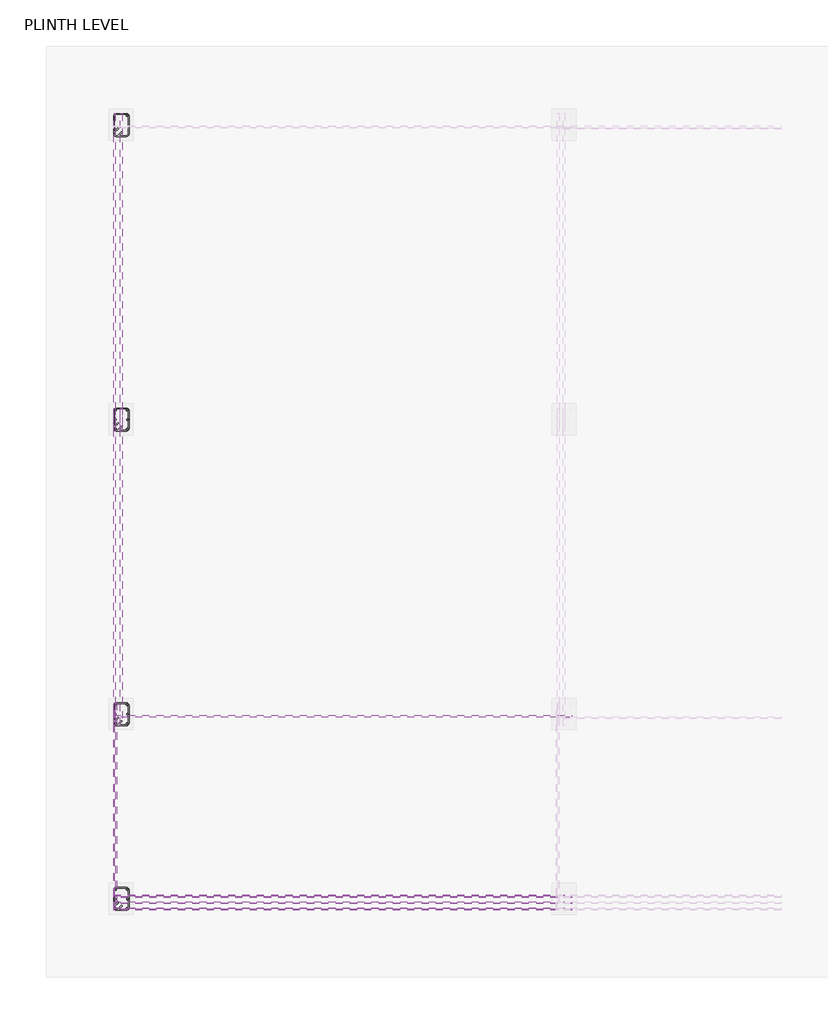
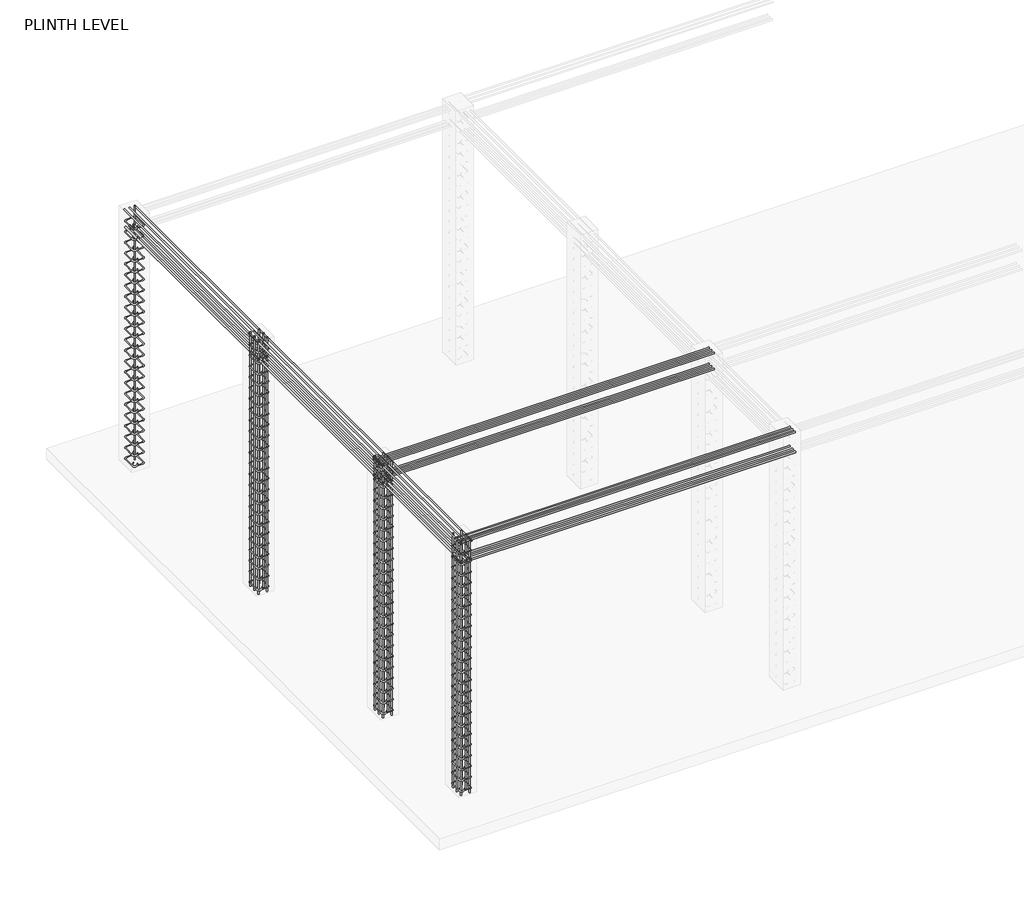
# One storey, part 2 of 6: 37 reinforcing bars.
"""IFC4 building model written with IfcOpenShell, lengths in millimetres."""

from ifc_helpers import new_model, si_unit, point, frame, origin, place, context, project, spatial, polyline, circle_curve, trimmed, segment, composite_curve, source, transform, mapped, element, save
from ifc_brep_helpers import swept_disk

model = new_model("IFC4")

# Units and contexts
model_context = context("Model", 3, world=origin())
ifc_project = project(units=[si_unit("LENGTHUNIT", "METRE", prefix="MILLI")], contexts=[model_context])

# Site, building, storey
site = spatial("IfcSite", under=ifc_project)
building = spatial("IfcBuilding", under=site)
storey = spatial("IfcBuildingStorey", under=building, Name="PLINTH LEVEL", Elevation=0.0)

# Reinforcing bars
placement = place(None, origin())
reinforcing_bar_shape = source(origin(), model_context, "Body", "SolidModel", [
    swept_disk(composite_curve([segment(polyline([(-2649.751223, -15125.7150493, 44.0), (-2683.6923485, -15159.6561748, 44.0)]), True, "CONTINUOUS"), segment(trimmed(circle_curve(frame((-2666.7217857, -15176.6267376, 44.0), z_axis=(0.0, 0.0, 1.0), x_axis=(-16.970562800000152, 16.970562799999243, 0.0)), 24.0), [point((-2683.6923485, -15159.6561748, 44.0))], [point((-2666.7217857, -15200.6267376, 44.0))], True, "CARTESIAN"), True, "CONTINUOUS"), segment(polyline([(-2666.7217857, -15200.6267376, 44.0), (-2572.7217857, -15200.6267376, 44.0)]), True, "CONTINUOUS"), segment(trimmed(circle_curve(frame((-2572.7217857, -15176.6267376, 44.0), z_axis=(0.0, 0.0, 1.0), x_axis=(0.0, -24.0, 0.0)), 24.0), [point((-2572.7217857, -15200.6267376, 44.0))], [point((-2548.7217857, -15176.6267376, 44.0))], True, "CARTESIAN"), True, "CONTINUOUS"), segment(polyline([(-2548.7217857, -15176.6267376, 44.0), (-2548.7217857, -15012.6267376, 44.0)]), True, "CONTINUOUS"), segment(trimmed(circle_curve(frame((-2572.6837885, -15012.6267376, 42.650028), z_axis=(-0.05624883273897079, 0.0, 0.9984167811167355), x_axis=(23.962002799999937, 0.0, 1.349972000000001)), 24.0), [point((-2548.7217857, -15012.6267376, 44.0))], [point((-2572.6837885, -14988.6267376, 42.650028))], True, "CARTESIAN"), True, "CONTINUOUS"), segment(polyline([(-2572.6837885, -14988.6267376, 42.650028), (-2666.759783, -14988.6267376, 37.349972)]), True, "CONTINUOUS"), segment(trimmed(circle_curve(frame((-2666.759783, -15012.6267376, 37.349972), z_axis=(-0.05624883273897079, 0.0, 0.9984167811167355), x_axis=(0.0, 24.0, 0.0)), 24.0), [point((-2666.759783, -14988.6267376, 37.349972))], [point((-2690.7217857, -15012.6267376, 36.0))], True, "CARTESIAN"), True, "CONTINUOUS"), segment(polyline([(-2690.7217857, -15012.6267376, 36.0), (-2690.7217857, -15176.6267376, 36.0)]), True, "CONTINUOUS"), segment(trimmed(circle_curve(frame((-2666.7217857, -15176.6267376, 36.0), z_axis=(0.0, 0.0, 1.0), x_axis=(-24.0, 0.0, 0.0)), 24.0), [point((-2690.7217857, -15176.6267376, 36.0))], [point((-2649.751223, -15193.5973003, 36.0))], True, "CARTESIAN"), True, "CONTINUOUS"), segment(polyline([(-2649.751223, -15193.5973003, 36.0), (-2615.8100975, -15159.6561748, 36.0)]), True, "CONTINUOUS")], self_intersect=False), 4.0),
])
element("IfcReinforcingBar", 1, at=placement, inside=storey, context=model_context, shape_type="MappedRepresentation", body=[
    mapped(reinforcing_bar_shape, transform((0.0, 0.0, 0.0), x_axis=(1.0, 0.0, 0.0), y_axis=(0.0, 1.0, 0.0), z_axis=(0.0, 0.0, 1.0))),
    mapped(reinforcing_bar_shape, transform((0.0, 0.0, 149.0483786), x_axis=(1.0, 0.0, 0.0), y_axis=(0.0, 1.0, 0.0), z_axis=(0.0, 0.0, 1.0))),
    mapped(reinforcing_bar_shape, transform((0.0, 0.0, 298.0967572), x_axis=(1.0, 0.0, 0.0), y_axis=(0.0, 1.0, 0.0), z_axis=(0.0, 0.0, 1.0))),
    mapped(reinforcing_bar_shape, transform((0.0, 0.0, 447.1451358), x_axis=(1.0, 0.0, 0.0), y_axis=(0.0, 1.0, 0.0), z_axis=(0.0, 0.0, 1.0))),
    mapped(reinforcing_bar_shape, transform((0.0, 0.0, 596.1935144), x_axis=(1.0, 0.0, 0.0), y_axis=(0.0, 1.0, 0.0), z_axis=(0.0, 0.0, 1.0))),
    mapped(reinforcing_bar_shape, transform((0.0, 0.0, 745.241893), x_axis=(1.0, 0.0, 0.0), y_axis=(0.0, 1.0, 0.0), z_axis=(0.0, 0.0, 1.0))),
    mapped(reinforcing_bar_shape, transform((0.0, 0.0, 894.2902717), x_axis=(1.0, 0.0, 0.0), y_axis=(0.0, 1.0, 0.0), z_axis=(0.0, 0.0, 1.0))),
    mapped(reinforcing_bar_shape, transform((0.0, 0.0, 1043.3386503), x_axis=(1.0, 0.0, 0.0), y_axis=(0.0, 1.0, 0.0), z_axis=(0.0, 0.0, 1.0))),
    mapped(reinforcing_bar_shape, transform((0.0, 0.0, 1192.3870289), x_axis=(1.0, 0.0, 0.0), y_axis=(0.0, 1.0, 0.0), z_axis=(0.0, 0.0, 1.0))),
    mapped(reinforcing_bar_shape, transform((0.0, 0.0, 1341.4354075), x_axis=(1.0, 0.0, 0.0), y_axis=(0.0, 1.0, 0.0), z_axis=(0.0, 0.0, 1.0))),
    mapped(reinforcing_bar_shape, transform((0.0, 0.0, 1490.4837861), x_axis=(1.0, 0.0, 0.0), y_axis=(0.0, 1.0, 0.0), z_axis=(0.0, 0.0, 1.0))),
    mapped(reinforcing_bar_shape, transform((0.0, 0.0, 1639.5321647), x_axis=(1.0, 0.0, 0.0), y_axis=(0.0, 1.0, 0.0), z_axis=(0.0, 0.0, 1.0))),
    mapped(reinforcing_bar_shape, transform((0.0, 0.0, 1788.5805433), x_axis=(1.0, 0.0, 0.0), y_axis=(0.0, 1.0, 0.0), z_axis=(0.0, 0.0, 1.0))),
    mapped(reinforcing_bar_shape, transform((0.0, 0.0, 1937.6289219), x_axis=(1.0, 0.0, 0.0), y_axis=(0.0, 1.0, 0.0), z_axis=(0.0, 0.0, 1.0))),
    mapped(reinforcing_bar_shape, transform((0.0, 0.0, 2086.6773005), x_axis=(1.0, 0.0, 0.0), y_axis=(0.0, 1.0, 0.0), z_axis=(0.0, 0.0, 1.0))),
    mapped(reinforcing_bar_shape, transform((0.0, 0.0, 2235.7256791), x_axis=(1.0, 0.0, 0.0), y_axis=(0.0, 1.0, 0.0), z_axis=(0.0, 0.0, 1.0))),
    mapped(reinforcing_bar_shape, transform((0.0, 0.0, 2384.7740578), x_axis=(1.0, 0.0, 0.0), y_axis=(0.0, 1.0, 0.0), z_axis=(0.0, 0.0, 1.0))),
    mapped(reinforcing_bar_shape, transform((0.0, 0.0, 2533.8224364), x_axis=(1.0, 0.0, 0.0), y_axis=(0.0, 1.0, 0.0), z_axis=(0.0, 0.0, 1.0))),
    mapped(reinforcing_bar_shape, transform((0.0, 0.0, 2682.870815), x_axis=(1.0, 0.0, 0.0), y_axis=(0.0, 1.0, 0.0), z_axis=(0.0, 0.0, 1.0))),
    mapped(reinforcing_bar_shape, transform((0.0, 0.0, 2831.9191936), x_axis=(1.0, 0.0, 0.0), y_axis=(0.0, 1.0, 0.0), z_axis=(0.0, 0.0, 1.0))),
    mapped(reinforcing_bar_shape, transform((0.0, 0.0, 2980.9675722), x_axis=(1.0, 0.0, 0.0), y_axis=(0.0, 1.0, 0.0), z_axis=(0.0, 0.0, 1.0))),
    mapped(reinforcing_bar_shape, transform((0.0, 0.0, 3130.0159508), x_axis=(1.0, 0.0, 0.0), y_axis=(0.0, 1.0, 0.0), z_axis=(0.0, 0.0, 1.0))),
    mapped(reinforcing_bar_shape, transform((0.0, 0.0, 3279.0643294), x_axis=(1.0, 0.0, 0.0), y_axis=(0.0, 1.0, 0.0), z_axis=(0.0, 0.0, 1.0))),
])
element("IfcReinforcingBar", 2, at=placement, inside=storey, context=model_context, shape_type="SolidModel", body=[
    swept_disk(composite_curve([segment(polyline([(-2564.2365043, -15004.1414562, -20.0), (-2564.2365043, -15004.1414562, 3485.2)]), True, "CONTINUOUS")], self_intersect=False), 8.0),
])
element("IfcReinforcingBar", 3, at=placement, inside=storey, context=model_context, shape_type="SolidModel", body=[
    swept_disk(composite_curve([segment(polyline([(-2564.2365043, -15185.112019, -20.0), (-2564.2365043, -15185.112019, 3485.2)]), True, "CONTINUOUS")], self_intersect=False), 8.0),
])
element("IfcReinforcingBar", 4, at=placement, inside=storey, context=model_context, shape_type="SolidModel", body=[
    swept_disk(composite_curve([segment(polyline([(-2560.7217857, -15094.6267376, -20.0), (-2560.7217857, -15094.6267376, 3485.2)]), True, "CONTINUOUS")], self_intersect=False), 8.0),
])
element("IfcReinforcingBar", 5, at=placement, inside=storey, context=model_context, shape_type="SolidModel", body=[
    swept_disk(composite_curve([segment(polyline([(-2675.2070671, -15004.1414562, -20.0), (-2675.2070671, -15004.1414562, 3485.2)]), True, "CONTINUOUS")], self_intersect=False), 8.0),
])
element("IfcReinforcingBar", 6, at=placement, inside=storey, context=model_context, shape_type="SolidModel", body=[
    swept_disk(composite_curve([segment(polyline([(-2675.2070671, -15185.112019, -20.0), (-2675.2070671, -15185.112019, 3485.2)]), True, "CONTINUOUS")], self_intersect=False), 8.0),
])
element("IfcReinforcingBar", 7, at=placement, inside=storey, context=model_context, shape_type="SolidModel", body=[
    swept_disk(composite_curve([segment(polyline([(-2678.7217857, -15094.6267376, -20.0), (-2678.7217857, -15094.6267376, 3485.2)]), True, "CONTINUOUS")], self_intersect=False), 8.0),
])
reinforcing_bar_2_shape = source(origin(), model_context, "Body", "SolidModel", [
    swept_disk(composite_curve([segment(polyline([(-2649.751223, -13360.7150493, 44.0), (-2683.6923485, -13394.6561748, 44.0)]), True, "CONTINUOUS"), segment(trimmed(circle_curve(frame((-2666.7217857, -13411.6267376, 44.0), z_axis=(0.0, 0.0, 1.0), x_axis=(-16.970562800000152, 16.970562799999243, 0.0)), 24.0), [point((-2683.6923485, -13394.6561748, 44.0))], [point((-2666.7217857, -13435.6267376, 44.0))], True, "CARTESIAN"), True, "CONTINUOUS"), segment(polyline([(-2666.7217857, -13435.6267376, 44.0), (-2572.7217857, -13435.6267376, 44.0)]), True, "CONTINUOUS"), segment(trimmed(circle_curve(frame((-2572.7217857, -13411.6267376, 44.0), z_axis=(0.0, 0.0, 1.0), x_axis=(0.0, -24.0, 0.0)), 24.0), [point((-2572.7217857, -13435.6267376, 44.0))], [point((-2548.7217857, -13411.6267376, 44.0))], True, "CARTESIAN"), True, "CONTINUOUS"), segment(polyline([(-2548.7217857, -13411.6267376, 44.0), (-2548.7217857, -13247.6267376, 44.0)]), True, "CONTINUOUS"), segment(trimmed(circle_curve(frame((-2572.6837885, -13247.6267376, 42.650028), z_axis=(-0.05624883273897079, 0.0, 0.9984167811167355), x_axis=(23.962002799999937, 0.0, 1.349972000000001)), 24.0), [point((-2548.7217857, -13247.6267376, 44.0))], [point((-2572.6837885, -13223.6267376, 42.650028))], True, "CARTESIAN"), True, "CONTINUOUS"), segment(polyline([(-2572.6837885, -13223.6267376, 42.650028), (-2666.759783, -13223.6267376, 37.349972)]), True, "CONTINUOUS"), segment(trimmed(circle_curve(frame((-2666.759783, -13247.6267376, 37.349972), z_axis=(-0.05624883273897079, 0.0, 0.9984167811167355), x_axis=(0.0, 24.0, 0.0)), 24.0), [point((-2666.759783, -13223.6267376, 37.349972))], [point((-2690.7217857, -13247.6267376, 36.0))], True, "CARTESIAN"), True, "CONTINUOUS"), segment(polyline([(-2690.7217857, -13247.6267376, 36.0), (-2690.7217857, -13411.6267376, 36.0)]), True, "CONTINUOUS"), segment(trimmed(circle_curve(frame((-2666.7217857, -13411.6267376, 36.0), z_axis=(0.0, 0.0, 1.0), x_axis=(-24.0, 0.0, 0.0)), 24.0), [point((-2690.7217857, -13411.6267376, 36.0))], [point((-2649.751223, -13428.5973003, 36.0))], True, "CARTESIAN"), True, "CONTINUOUS"), segment(polyline([(-2649.751223, -13428.5973003, 36.0), (-2615.8100975, -13394.6561748, 36.0)]), True, "CONTINUOUS")], self_intersect=False), 4.0),
])
element("IfcReinforcingBar", 8, at=placement, inside=storey, context=model_context, shape_type="MappedRepresentation", body=[
    mapped(reinforcing_bar_2_shape, transform((0.0, 0.0, 0.0), x_axis=(1.0, 0.0, 0.0), y_axis=(0.0, 1.0, 0.0), z_axis=(0.0, 0.0, 1.0))),
    mapped(reinforcing_bar_2_shape, transform((0.0, 0.0, 149.0483786), x_axis=(1.0, 0.0, 0.0), y_axis=(0.0, 1.0, 0.0), z_axis=(0.0, 0.0, 1.0))),
    mapped(reinforcing_bar_2_shape, transform((0.0, 0.0, 298.0967572), x_axis=(1.0, 0.0, 0.0), y_axis=(0.0, 1.0, 0.0), z_axis=(0.0, 0.0, 1.0))),
    mapped(reinforcing_bar_2_shape, transform((0.0, 0.0, 447.1451358), x_axis=(1.0, 0.0, 0.0), y_axis=(0.0, 1.0, 0.0), z_axis=(0.0, 0.0, 1.0))),
    mapped(reinforcing_bar_2_shape, transform((0.0, 0.0, 596.1935144), x_axis=(1.0, 0.0, 0.0), y_axis=(0.0, 1.0, 0.0), z_axis=(0.0, 0.0, 1.0))),
    mapped(reinforcing_bar_2_shape, transform((0.0, 0.0, 745.241893), x_axis=(1.0, 0.0, 0.0), y_axis=(0.0, 1.0, 0.0), z_axis=(0.0, 0.0, 1.0))),
    mapped(reinforcing_bar_2_shape, transform((0.0, 0.0, 894.2902717), x_axis=(1.0, 0.0, 0.0), y_axis=(0.0, 1.0, 0.0), z_axis=(0.0, 0.0, 1.0))),
    mapped(reinforcing_bar_2_shape, transform((0.0, 0.0, 1043.3386503), x_axis=(1.0, 0.0, 0.0), y_axis=(0.0, 1.0, 0.0), z_axis=(0.0, 0.0, 1.0))),
    mapped(reinforcing_bar_2_shape, transform((0.0, 0.0, 1192.3870289), x_axis=(1.0, 0.0, 0.0), y_axis=(0.0, 1.0, 0.0), z_axis=(0.0, 0.0, 1.0))),
    mapped(reinforcing_bar_2_shape, transform((0.0, 0.0, 1341.4354075), x_axis=(1.0, 0.0, 0.0), y_axis=(0.0, 1.0, 0.0), z_axis=(0.0, 0.0, 1.0))),
    mapped(reinforcing_bar_2_shape, transform((0.0, 0.0, 1490.4837861), x_axis=(1.0, 0.0, 0.0), y_axis=(0.0, 1.0, 0.0), z_axis=(0.0, 0.0, 1.0))),
    mapped(reinforcing_bar_2_shape, transform((0.0, 0.0, 1639.5321647), x_axis=(1.0, 0.0, 0.0), y_axis=(0.0, 1.0, 0.0), z_axis=(0.0, 0.0, 1.0))),
    mapped(reinforcing_bar_2_shape, transform((0.0, 0.0, 1788.5805433), x_axis=(1.0, 0.0, 0.0), y_axis=(0.0, 1.0, 0.0), z_axis=(0.0, 0.0, 1.0))),
    mapped(reinforcing_bar_2_shape, transform((0.0, 0.0, 1937.6289219), x_axis=(1.0, 0.0, 0.0), y_axis=(0.0, 1.0, 0.0), z_axis=(0.0, 0.0, 1.0))),
    mapped(reinforcing_bar_2_shape, transform((0.0, 0.0, 2086.6773005), x_axis=(1.0, 0.0, 0.0), y_axis=(0.0, 1.0, 0.0), z_axis=(0.0, 0.0, 1.0))),
    mapped(reinforcing_bar_2_shape, transform((0.0, 0.0, 2235.7256791), x_axis=(1.0, 0.0, 0.0), y_axis=(0.0, 1.0, 0.0), z_axis=(0.0, 0.0, 1.0))),
    mapped(reinforcing_bar_2_shape, transform((0.0, 0.0, 2384.7740578), x_axis=(1.0, 0.0, 0.0), y_axis=(0.0, 1.0, 0.0), z_axis=(0.0, 0.0, 1.0))),
    mapped(reinforcing_bar_2_shape, transform((0.0, 0.0, 2533.8224364), x_axis=(1.0, 0.0, 0.0), y_axis=(0.0, 1.0, 0.0), z_axis=(0.0, 0.0, 1.0))),
    mapped(reinforcing_bar_2_shape, transform((0.0, 0.0, 2682.870815), x_axis=(1.0, 0.0, 0.0), y_axis=(0.0, 1.0, 0.0), z_axis=(0.0, 0.0, 1.0))),
    mapped(reinforcing_bar_2_shape, transform((0.0, 0.0, 2831.9191936), x_axis=(1.0, 0.0, 0.0), y_axis=(0.0, 1.0, 0.0), z_axis=(0.0, 0.0, 1.0))),
    mapped(reinforcing_bar_2_shape, transform((0.0, 0.0, 2980.9675722), x_axis=(1.0, 0.0, 0.0), y_axis=(0.0, 1.0, 0.0), z_axis=(0.0, 0.0, 1.0))),
    mapped(reinforcing_bar_2_shape, transform((0.0, 0.0, 3130.0159508), x_axis=(1.0, 0.0, 0.0), y_axis=(0.0, 1.0, 0.0), z_axis=(0.0, 0.0, 1.0))),
    mapped(reinforcing_bar_2_shape, transform((0.0, 0.0, 3279.0643294), x_axis=(1.0, 0.0, 0.0), y_axis=(0.0, 1.0, 0.0), z_axis=(0.0, 0.0, 1.0))),
])
element("IfcReinforcingBar", 9, at=placement, inside=storey, context=model_context, shape_type="SolidModel", body=[
    swept_disk(composite_curve([segment(polyline([(-2564.2365043, -13239.1414562, -20.0), (-2564.2365043, -13239.1414562, 3485.2)]), True, "CONTINUOUS")], self_intersect=False), 8.0),
])
element("IfcReinforcingBar", 10, at=placement, inside=storey, context=model_context, shape_type="SolidModel", body=[
    swept_disk(composite_curve([segment(polyline([(-2564.2365043, -13420.112019, -20.0), (-2564.2365043, -13420.112019, 3485.2)]), True, "CONTINUOUS")], self_intersect=False), 8.0),
])
element("IfcReinforcingBar", 11, at=placement, inside=storey, context=model_context, shape_type="SolidModel", body=[
    swept_disk(composite_curve([segment(polyline([(-2560.7217857, -13329.6267376, -20.0), (-2560.7217857, -13329.6267376, 3485.2)]), True, "CONTINUOUS")], self_intersect=False), 8.0),
])
element("IfcReinforcingBar", 12, at=placement, inside=storey, context=model_context, shape_type="SolidModel", body=[
    swept_disk(composite_curve([segment(polyline([(-2675.2070671, -13239.1414562, -20.0), (-2675.2070671, -13239.1414562, 3485.2)]), True, "CONTINUOUS")], self_intersect=False), 8.0),
])
element("IfcReinforcingBar", 13, at=placement, inside=storey, context=model_context, shape_type="SolidModel", body=[
    swept_disk(composite_curve([segment(polyline([(-2675.2070671, -13420.112019, -20.0), (-2675.2070671, -13420.112019, 3485.2)]), True, "CONTINUOUS")], self_intersect=False), 8.0),
])
element("IfcReinforcingBar", 14, at=placement, inside=storey, context=model_context, shape_type="SolidModel", body=[
    swept_disk(composite_curve([segment(polyline([(-2678.7217857, -13329.6267376, -20.0), (-2678.7217857, -13329.6267376, 3485.2)]), True, "CONTINUOUS")], self_intersect=False), 8.0),
])
reinforcing_bar_3_shape = source(origin(), model_context, "Body", "SolidModel", [
    swept_disk(composite_curve([segment(polyline([(-2649.751223, -10545.7150493, 44.0), (-2683.6923485, -10579.6561748, 44.0)]), True, "CONTINUOUS"), segment(trimmed(circle_curve(frame((-2666.7217857, -10596.6267376, 44.0), z_axis=(0.0, 0.0, 1.0), x_axis=(-16.970562800000152, 16.970562799999243, 0.0)), 24.0), [point((-2683.6923485, -10579.6561748, 44.0))], [point((-2666.7217857, -10620.6267376, 44.0))], True, "CARTESIAN"), True, "CONTINUOUS"), segment(polyline([(-2666.7217857, -10620.6267376, 44.0), (-2572.7217857, -10620.6267376, 44.0)]), True, "CONTINUOUS"), segment(trimmed(circle_curve(frame((-2572.7217857, -10596.6267376, 44.0), z_axis=(0.0, 0.0, 1.0), x_axis=(0.0, -24.0, 0.0)), 24.0), [point((-2572.7217857, -10620.6267376, 44.0))], [point((-2548.7217857, -10596.6267376, 44.0))], True, "CARTESIAN"), True, "CONTINUOUS"), segment(polyline([(-2548.7217857, -10596.6267376, 44.0), (-2548.7217857, -10432.6267376, 44.0)]), True, "CONTINUOUS"), segment(trimmed(circle_curve(frame((-2572.6837885, -10432.6267376, 42.650028), z_axis=(-0.05624883273897079, 0.0, 0.9984167811167355), x_axis=(23.962002799999937, 0.0, 1.349972000000001)), 24.0), [point((-2548.7217857, -10432.6267376, 44.0))], [point((-2572.6837885, -10408.6267376, 42.650028))], True, "CARTESIAN"), True, "CONTINUOUS"), segment(polyline([(-2572.6837885, -10408.6267376, 42.650028), (-2666.759783, -10408.6267376, 37.349972)]), True, "CONTINUOUS"), segment(trimmed(circle_curve(frame((-2666.759783, -10432.6267376, 37.349972), z_axis=(-0.05624883273897079, 0.0, 0.9984167811167355), x_axis=(0.0, 24.0, 0.0)), 24.0), [point((-2666.759783, -10408.6267376, 37.349972))], [point((-2690.7217857, -10432.6267376, 36.0))], True, "CARTESIAN"), True, "CONTINUOUS"), segment(polyline([(-2690.7217857, -10432.6267376, 36.0), (-2690.7217857, -10596.6267376, 36.0)]), True, "CONTINUOUS"), segment(trimmed(circle_curve(frame((-2666.7217857, -10596.6267376, 36.0), z_axis=(0.0, 0.0, 1.0), x_axis=(-24.0, 0.0, 0.0)), 24.0), [point((-2690.7217857, -10596.6267376, 36.0))], [point((-2649.751223, -10613.5973003, 36.0))], True, "CARTESIAN"), True, "CONTINUOUS"), segment(polyline([(-2649.751223, -10613.5973003, 36.0), (-2615.8100975, -10579.6561748, 36.0)]), True, "CONTINUOUS")], self_intersect=False), 4.0),
])
element("IfcReinforcingBar", 15, at=placement, inside=storey, context=model_context, shape_type="MappedRepresentation", body=[
    mapped(reinforcing_bar_3_shape, transform((0.0, 0.0, 0.0), x_axis=(1.0, 0.0, 0.0), y_axis=(0.0, 1.0, 0.0), z_axis=(0.0, 0.0, 1.0))),
    mapped(reinforcing_bar_3_shape, transform((0.0, 0.0, 149.0483786), x_axis=(1.0, 0.0, 0.0), y_axis=(0.0, 1.0, 0.0), z_axis=(0.0, 0.0, 1.0))),
    mapped(reinforcing_bar_3_shape, transform((0.0, 0.0, 298.0967572), x_axis=(1.0, 0.0, 0.0), y_axis=(0.0, 1.0, 0.0), z_axis=(0.0, 0.0, 1.0))),
    mapped(reinforcing_bar_3_shape, transform((0.0, 0.0, 447.1451358), x_axis=(1.0, 0.0, 0.0), y_axis=(0.0, 1.0, 0.0), z_axis=(0.0, 0.0, 1.0))),
    mapped(reinforcing_bar_3_shape, transform((0.0, 0.0, 596.1935144), x_axis=(1.0, 0.0, 0.0), y_axis=(0.0, 1.0, 0.0), z_axis=(0.0, 0.0, 1.0))),
    mapped(reinforcing_bar_3_shape, transform((0.0, 0.0, 745.241893), x_axis=(1.0, 0.0, 0.0), y_axis=(0.0, 1.0, 0.0), z_axis=(0.0, 0.0, 1.0))),
    mapped(reinforcing_bar_3_shape, transform((0.0, 0.0, 894.2902717), x_axis=(1.0, 0.0, 0.0), y_axis=(0.0, 1.0, 0.0), z_axis=(0.0, 0.0, 1.0))),
    mapped(reinforcing_bar_3_shape, transform((0.0, 0.0, 1043.3386503), x_axis=(1.0, 0.0, 0.0), y_axis=(0.0, 1.0, 0.0), z_axis=(0.0, 0.0, 1.0))),
    mapped(reinforcing_bar_3_shape, transform((0.0, 0.0, 1192.3870289), x_axis=(1.0, 0.0, 0.0), y_axis=(0.0, 1.0, 0.0), z_axis=(0.0, 0.0, 1.0))),
    mapped(reinforcing_bar_3_shape, transform((0.0, 0.0, 1341.4354075), x_axis=(1.0, 0.0, 0.0), y_axis=(0.0, 1.0, 0.0), z_axis=(0.0, 0.0, 1.0))),
    mapped(reinforcing_bar_3_shape, transform((0.0, 0.0, 1490.4837861), x_axis=(1.0, 0.0, 0.0), y_axis=(0.0, 1.0, 0.0), z_axis=(0.0, 0.0, 1.0))),
    mapped(reinforcing_bar_3_shape, transform((0.0, 0.0, 1639.5321647), x_axis=(1.0, 0.0, 0.0), y_axis=(0.0, 1.0, 0.0), z_axis=(0.0, 0.0, 1.0))),
    mapped(reinforcing_bar_3_shape, transform((0.0, 0.0, 1788.5805433), x_axis=(1.0, 0.0, 0.0), y_axis=(0.0, 1.0, 0.0), z_axis=(0.0, 0.0, 1.0))),
    mapped(reinforcing_bar_3_shape, transform((0.0, 0.0, 1937.6289219), x_axis=(1.0, 0.0, 0.0), y_axis=(0.0, 1.0, 0.0), z_axis=(0.0, 0.0, 1.0))),
    mapped(reinforcing_bar_3_shape, transform((0.0, 0.0, 2086.6773005), x_axis=(1.0, 0.0, 0.0), y_axis=(0.0, 1.0, 0.0), z_axis=(0.0, 0.0, 1.0))),
    mapped(reinforcing_bar_3_shape, transform((0.0, 0.0, 2235.7256791), x_axis=(1.0, 0.0, 0.0), y_axis=(0.0, 1.0, 0.0), z_axis=(0.0, 0.0, 1.0))),
    mapped(reinforcing_bar_3_shape, transform((0.0, 0.0, 2384.7740578), x_axis=(1.0, 0.0, 0.0), y_axis=(0.0, 1.0, 0.0), z_axis=(0.0, 0.0, 1.0))),
    mapped(reinforcing_bar_3_shape, transform((0.0, 0.0, 2533.8224364), x_axis=(1.0, 0.0, 0.0), y_axis=(0.0, 1.0, 0.0), z_axis=(0.0, 0.0, 1.0))),
    mapped(reinforcing_bar_3_shape, transform((0.0, 0.0, 2682.870815), x_axis=(1.0, 0.0, 0.0), y_axis=(0.0, 1.0, 0.0), z_axis=(0.0, 0.0, 1.0))),
    mapped(reinforcing_bar_3_shape, transform((0.0, 0.0, 2831.9191936), x_axis=(1.0, 0.0, 0.0), y_axis=(0.0, 1.0, 0.0), z_axis=(0.0, 0.0, 1.0))),
    mapped(reinforcing_bar_3_shape, transform((0.0, 0.0, 2980.9675722), x_axis=(1.0, 0.0, 0.0), y_axis=(0.0, 1.0, 0.0), z_axis=(0.0, 0.0, 1.0))),
    mapped(reinforcing_bar_3_shape, transform((0.0, 0.0, 3130.0159508), x_axis=(1.0, 0.0, 0.0), y_axis=(0.0, 1.0, 0.0), z_axis=(0.0, 0.0, 1.0))),
    mapped(reinforcing_bar_3_shape, transform((0.0, 0.0, 3279.0643294), x_axis=(1.0, 0.0, 0.0), y_axis=(0.0, 1.0, 0.0), z_axis=(0.0, 0.0, 1.0))),
])
element("IfcReinforcingBar", 16, at=placement, inside=storey, context=model_context, shape_type="SolidModel", body=[
    swept_disk(composite_curve([segment(polyline([(-2564.2365043, -10424.1414562, -20.0), (-2564.2365043, -10424.1414562, 3485.2)]), True, "CONTINUOUS")], self_intersect=False), 8.0),
])
element("IfcReinforcingBar", 17, at=placement, inside=storey, context=model_context, shape_type="SolidModel", body=[
    swept_disk(composite_curve([segment(polyline([(-2564.2365043, -10605.112019, -20.0), (-2564.2365043, -10605.112019, 3485.2)]), True, "CONTINUOUS")], self_intersect=False), 8.0),
])
element("IfcReinforcingBar", 18, at=placement, inside=storey, context=model_context, shape_type="SolidModel", body=[
    swept_disk(composite_curve([segment(polyline([(-2560.7217857, -10514.6267376, -20.0), (-2560.7217857, -10514.6267376, 3485.2)]), True, "CONTINUOUS")], self_intersect=False), 8.0),
])
element("IfcReinforcingBar", 19, at=placement, inside=storey, context=model_context, shape_type="SolidModel", body=[
    swept_disk(composite_curve([segment(polyline([(-2675.2070671, -10424.1414562, -20.0), (-2675.2070671, -10424.1414562, 3485.2)]), True, "CONTINUOUS")], self_intersect=False), 8.0),
])
element("IfcReinforcingBar", 20, at=placement, inside=storey, context=model_context, shape_type="SolidModel", body=[
    swept_disk(composite_curve([segment(polyline([(-2675.2070671, -10605.112019, -20.0), (-2675.2070671, -10605.112019, 3485.2)]), True, "CONTINUOUS")], self_intersect=False), 8.0),
])
element("IfcReinforcingBar", 21, at=placement, inside=storey, context=model_context, shape_type="SolidModel", body=[
    swept_disk(composite_curve([segment(polyline([(-2678.7217857, -10514.6267376, -20.0), (-2678.7217857, -10514.6267376, 3485.2)]), True, "CONTINUOUS")], self_intersect=False), 8.0),
])
reinforcing_bar_4_shape = source(origin(), model_context, "Body", "SolidModel", [
    swept_disk(composite_curve([segment(polyline([(-2649.751223, -7730.7150493, 44.0), (-2683.6923485, -7764.6561748, 44.0)]), True, "CONTINUOUS"), segment(trimmed(circle_curve(frame((-2666.7217857, -7781.6267376, 44.0), z_axis=(0.0, 0.0, 1.0), x_axis=(-16.970562800000152, 16.970562799999243, 0.0)), 24.0), [point((-2683.6923485, -7764.6561748, 44.0))], [point((-2666.7217857, -7805.6267376, 44.0))], True, "CARTESIAN"), True, "CONTINUOUS"), segment(polyline([(-2666.7217857, -7805.6267376, 44.0), (-2572.7217857, -7805.6267376, 44.0)]), True, "CONTINUOUS"), segment(trimmed(circle_curve(frame((-2572.7217857, -7781.6267376, 44.0), z_axis=(0.0, 0.0, 1.0), x_axis=(0.0, -24.0, 0.0)), 24.0), [point((-2572.7217857, -7805.6267376, 44.0))], [point((-2548.7217857, -7781.6267376, 44.0))], True, "CARTESIAN"), True, "CONTINUOUS"), segment(polyline([(-2548.7217857, -7781.6267376, 44.0), (-2548.7217857, -7617.6267376, 44.0)]), True, "CONTINUOUS"), segment(trimmed(circle_curve(frame((-2572.6837885, -7617.6267376, 42.650028), z_axis=(-0.05624883273897079, 0.0, 0.9984167811167355), x_axis=(23.962002799999937, 0.0, 1.349972000000001)), 24.0), [point((-2548.7217857, -7617.6267376, 44.0))], [point((-2572.6837885, -7593.6267376, 42.650028))], True, "CARTESIAN"), True, "CONTINUOUS"), segment(polyline([(-2572.6837885, -7593.6267376, 42.650028), (-2666.759783, -7593.6267376, 37.349972)]), True, "CONTINUOUS"), segment(trimmed(circle_curve(frame((-2666.759783, -7617.6267376, 37.349972), z_axis=(-0.05624883273897079, 0.0, 0.9984167811167355), x_axis=(0.0, 24.0, 0.0)), 24.0), [point((-2666.759783, -7593.6267376, 37.349972))], [point((-2690.7217857, -7617.6267376, 36.0))], True, "CARTESIAN"), True, "CONTINUOUS"), segment(polyline([(-2690.7217857, -7617.6267376, 36.0), (-2690.7217857, -7781.6267376, 36.0)]), True, "CONTINUOUS"), segment(trimmed(circle_curve(frame((-2666.7217857, -7781.6267376, 36.0), z_axis=(0.0, 0.0, 1.0), x_axis=(-24.0, 0.0, 0.0)), 24.0), [point((-2690.7217857, -7781.6267376, 36.0))], [point((-2649.751223, -7798.5973003, 36.0))], True, "CARTESIAN"), True, "CONTINUOUS"), segment(polyline([(-2649.751223, -7798.5973003, 36.0), (-2615.8100975, -7764.6561748, 36.0)]), True, "CONTINUOUS")], self_intersect=False), 4.0),
])
element("IfcReinforcingBar", 22, at=placement, inside=storey, context=model_context, shape_type="MappedRepresentation", body=[
    mapped(reinforcing_bar_4_shape, transform((0.0, 0.0, 0.0), x_axis=(1.0, 0.0, 0.0), y_axis=(0.0, 1.0, 0.0), z_axis=(0.0, 0.0, 1.0))),
    mapped(reinforcing_bar_4_shape, transform((0.0, 0.0, 149.0483786), x_axis=(1.0, 0.0, 0.0), y_axis=(0.0, 1.0, 0.0), z_axis=(0.0, 0.0, 1.0))),
    mapped(reinforcing_bar_4_shape, transform((0.0, 0.0, 298.0967572), x_axis=(1.0, 0.0, 0.0), y_axis=(0.0, 1.0, 0.0), z_axis=(0.0, 0.0, 1.0))),
    mapped(reinforcing_bar_4_shape, transform((0.0, 0.0, 447.1451358), x_axis=(1.0, 0.0, 0.0), y_axis=(0.0, 1.0, 0.0), z_axis=(0.0, 0.0, 1.0))),
    mapped(reinforcing_bar_4_shape, transform((0.0, 0.0, 596.1935144), x_axis=(1.0, 0.0, 0.0), y_axis=(0.0, 1.0, 0.0), z_axis=(0.0, 0.0, 1.0))),
    mapped(reinforcing_bar_4_shape, transform((0.0, 0.0, 745.241893), x_axis=(1.0, 0.0, 0.0), y_axis=(0.0, 1.0, 0.0), z_axis=(0.0, 0.0, 1.0))),
    mapped(reinforcing_bar_4_shape, transform((0.0, 0.0, 894.2902717), x_axis=(1.0, 0.0, 0.0), y_axis=(0.0, 1.0, 0.0), z_axis=(0.0, 0.0, 1.0))),
    mapped(reinforcing_bar_4_shape, transform((0.0, 0.0, 1043.3386503), x_axis=(1.0, 0.0, 0.0), y_axis=(0.0, 1.0, 0.0), z_axis=(0.0, 0.0, 1.0))),
    mapped(reinforcing_bar_4_shape, transform((0.0, 0.0, 1192.3870289), x_axis=(1.0, 0.0, 0.0), y_axis=(0.0, 1.0, 0.0), z_axis=(0.0, 0.0, 1.0))),
    mapped(reinforcing_bar_4_shape, transform((0.0, 0.0, 1341.4354075), x_axis=(1.0, 0.0, 0.0), y_axis=(0.0, 1.0, 0.0), z_axis=(0.0, 0.0, 1.0))),
    mapped(reinforcing_bar_4_shape, transform((0.0, 0.0, 1490.4837861), x_axis=(1.0, 0.0, 0.0), y_axis=(0.0, 1.0, 0.0), z_axis=(0.0, 0.0, 1.0))),
    mapped(reinforcing_bar_4_shape, transform((0.0, 0.0, 1639.5321647), x_axis=(1.0, 0.0, 0.0), y_axis=(0.0, 1.0, 0.0), z_axis=(0.0, 0.0, 1.0))),
    mapped(reinforcing_bar_4_shape, transform((0.0, 0.0, 1788.5805433), x_axis=(1.0, 0.0, 0.0), y_axis=(0.0, 1.0, 0.0), z_axis=(0.0, 0.0, 1.0))),
    mapped(reinforcing_bar_4_shape, transform((0.0, 0.0, 1937.6289219), x_axis=(1.0, 0.0, 0.0), y_axis=(0.0, 1.0, 0.0), z_axis=(0.0, 0.0, 1.0))),
    mapped(reinforcing_bar_4_shape, transform((0.0, 0.0, 2086.6773005), x_axis=(1.0, 0.0, 0.0), y_axis=(0.0, 1.0, 0.0), z_axis=(0.0, 0.0, 1.0))),
    mapped(reinforcing_bar_4_shape, transform((0.0, 0.0, 2235.7256791), x_axis=(1.0, 0.0, 0.0), y_axis=(0.0, 1.0, 0.0), z_axis=(0.0, 0.0, 1.0))),
    mapped(reinforcing_bar_4_shape, transform((0.0, 0.0, 2384.7740578), x_axis=(1.0, 0.0, 0.0), y_axis=(0.0, 1.0, 0.0), z_axis=(0.0, 0.0, 1.0))),
    mapped(reinforcing_bar_4_shape, transform((0.0, 0.0, 2533.8224364), x_axis=(1.0, 0.0, 0.0), y_axis=(0.0, 1.0, 0.0), z_axis=(0.0, 0.0, 1.0))),
    mapped(reinforcing_bar_4_shape, transform((0.0, 0.0, 2682.870815), x_axis=(1.0, 0.0, 0.0), y_axis=(0.0, 1.0, 0.0), z_axis=(0.0, 0.0, 1.0))),
    mapped(reinforcing_bar_4_shape, transform((0.0, 0.0, 2831.9191936), x_axis=(1.0, 0.0, 0.0), y_axis=(0.0, 1.0, 0.0), z_axis=(0.0, 0.0, 1.0))),
    mapped(reinforcing_bar_4_shape, transform((0.0, 0.0, 2980.9675722), x_axis=(1.0, 0.0, 0.0), y_axis=(0.0, 1.0, 0.0), z_axis=(0.0, 0.0, 1.0))),
    mapped(reinforcing_bar_4_shape, transform((0.0, 0.0, 3130.0159508), x_axis=(1.0, 0.0, 0.0), y_axis=(0.0, 1.0, 0.0), z_axis=(0.0, 0.0, 1.0))),
    mapped(reinforcing_bar_4_shape, transform((0.0, 0.0, 3279.0643294), x_axis=(1.0, 0.0, 0.0), y_axis=(0.0, 1.0, 0.0), z_axis=(0.0, 0.0, 1.0))),
])
element("IfcReinforcingBar", 23, at=placement, inside=storey, context=model_context, shape_type="SolidModel", body=[
    swept_disk(composite_curve([segment(polyline([(-2564.2365043, -7609.1414562, -20.0), (-2564.2365043, -7609.1414562, 3485.2)]), True, "CONTINUOUS")], self_intersect=False), 8.0),
])
reinforcing_bar_5_shape = source(origin(), model_context, "Body", "SolidModel", [
    swept_disk(composite_curve([segment(polyline([(-2552.7217857, -7589.6267376, 3463.45), (-2552.7217857, -10624.6267376, 3463.45)]), True, "CONTINUOUS")], self_intersect=False), 8.0),
])
element("IfcReinforcingBar", 24, at=placement, inside=storey, context=model_context, shape_type="MappedRepresentation", body=[
    mapped(reinforcing_bar_5_shape, transform((0.0, 0.0, 0.0), x_axis=(1.0, 0.0, 0.0), y_axis=(0.0, 1.0, 0.0), z_axis=(0.0, 0.0, 1.0))),
    mapped(reinforcing_bar_5_shape, transform((-67.0, 0.0, 0.0), x_axis=(1.0, 0.0, 0.0), y_axis=(0.0, 1.0, 0.0), z_axis=(0.0, 0.0, 1.0))),
    mapped(reinforcing_bar_5_shape, transform((-134.0, 0.0, 0.0), x_axis=(1.0, 0.0, 0.0), y_axis=(0.0, 1.0, 0.0), z_axis=(0.0, 0.0, 1.0))),
])
reinforcing_bar_6_shape = source(origin(), model_context, "Body", "SolidModel", [
    swept_disk(composite_curve([segment(polyline([(-2673.7928535, -7589.6267376, 3216.1289322), (-2673.7928535, -10624.6267376, 3216.1289322)]), True, "CONTINUOUS")], self_intersect=False), 10.0),
])
element("IfcReinforcingBar", 25, at=placement, inside=storey, context=model_context, shape_type="MappedRepresentation", body=[
    mapped(reinforcing_bar_6_shape, transform((0.0, 0.0, 0.0), x_axis=(1.0, 0.0, 0.0), y_axis=(0.0, 1.0, 0.0), z_axis=(0.0, 0.0, 1.0))),
    mapped(reinforcing_bar_6_shape, transform((54.0710678, 0.0, 0.0), x_axis=(1.0, 0.0, 0.0), y_axis=(0.0, 1.0, 0.0), z_axis=(0.0, 0.0, 1.0))),
    mapped(reinforcing_bar_6_shape, transform((108.1421356, 0.0, 0.0), x_axis=(1.0, 0.0, 0.0), y_axis=(0.0, 1.0, 0.0), z_axis=(0.0, 0.0, 1.0))),
])
reinforcing_bar_7_shape = source(origin(), model_context, "Body", "SolidModel", [
    swept_disk(composite_curve([segment(polyline([(-2552.7217857, -10404.6267376, 3463.45), (-2552.7217857, -13439.6267376, 3463.45)]), True, "CONTINUOUS")], self_intersect=False), 8.0),
])
element("IfcReinforcingBar", 26, at=placement, inside=storey, context=model_context, shape_type="MappedRepresentation", body=[
    mapped(reinforcing_bar_7_shape, transform((0.0, 0.0, 0.0), x_axis=(1.0, 0.0, 0.0), y_axis=(0.0, 1.0, 0.0), z_axis=(0.0, 0.0, 1.0))),
    mapped(reinforcing_bar_7_shape, transform((-67.0, 0.0, 0.0), x_axis=(1.0, 0.0, 0.0), y_axis=(0.0, 1.0, 0.0), z_axis=(0.0, 0.0, 1.0))),
    mapped(reinforcing_bar_7_shape, transform((-134.0, 0.0, 0.0), x_axis=(1.0, 0.0, 0.0), y_axis=(0.0, 1.0, 0.0), z_axis=(0.0, 0.0, 1.0))),
])
reinforcing_bar_8_shape = source(origin(), model_context, "Body", "SolidModel", [
    swept_disk(composite_curve([segment(polyline([(-2673.7928535, -10404.6267376, 3216.1289322), (-2673.7928535, -13439.6267376, 3216.1289322)]), True, "CONTINUOUS")], self_intersect=False), 10.0),
])
element("IfcReinforcingBar", 27, at=placement, inside=storey, context=model_context, shape_type="MappedRepresentation", body=[
    mapped(reinforcing_bar_8_shape, transform((0.0, 0.0, 0.0), x_axis=(1.0, 0.0, 0.0), y_axis=(0.0, 1.0, 0.0), z_axis=(0.0, 0.0, 1.0))),
    mapped(reinforcing_bar_8_shape, transform((54.0710678, 0.0, 0.0), x_axis=(1.0, 0.0, 0.0), y_axis=(0.0, 1.0, 0.0), z_axis=(0.0, 0.0, 1.0))),
    mapped(reinforcing_bar_8_shape, transform((108.1421356, 0.0, 0.0), x_axis=(1.0, 0.0, 0.0), y_axis=(0.0, 1.0, 0.0), z_axis=(0.0, 0.0, 1.0))),
])
reinforcing_bar_9_shape = source(origin(), model_context, "Body", "SolidModel", [
    swept_disk(composite_curve([segment(polyline([(-2552.7217857, -13219.6267376, 3463.45), (-2552.7217857, -15204.6267376, 3463.45)]), True, "CONTINUOUS")], self_intersect=False), 8.0),
])
element("IfcReinforcingBar", 28, at=placement, inside=storey, context=model_context, shape_type="MappedRepresentation", body=[
    mapped(reinforcing_bar_9_shape, transform((0.0, 0.0, 0.0), x_axis=(1.0, 0.0, 0.0), y_axis=(0.0, 1.0, 0.0), z_axis=(0.0, 0.0, 1.0))),
    mapped(reinforcing_bar_9_shape, transform((-67.0, 0.0, 0.0), x_axis=(1.0, 0.0, 0.0), y_axis=(0.0, 1.0, 0.0), z_axis=(0.0, 0.0, 1.0))),
    mapped(reinforcing_bar_9_shape, transform((-134.0, 0.0, 0.0), x_axis=(1.0, 0.0, 0.0), y_axis=(0.0, 1.0, 0.0), z_axis=(0.0, 0.0, 1.0))),
])
reinforcing_bar_10_shape = source(origin(), model_context, "Body", "SolidModel", [
    swept_disk(composite_curve([segment(polyline([(-2673.7928535, -13219.6267376, 3216.1289322), (-2673.7928535, -15204.6267376, 3216.1289322)]), True, "CONTINUOUS")], self_intersect=False), 10.0),
])
element("IfcReinforcingBar", 29, at=placement, inside=storey, context=model_context, shape_type="MappedRepresentation", body=[
    mapped(reinforcing_bar_10_shape, transform((0.0, 0.0, 0.0), x_axis=(1.0, 0.0, 0.0), y_axis=(0.0, 1.0, 0.0), z_axis=(0.0, 0.0, 1.0))),
    mapped(reinforcing_bar_10_shape, transform((54.0710678, 0.0, 0.0), x_axis=(1.0, 0.0, 0.0), y_axis=(0.0, 1.0, 0.0), z_axis=(0.0, 0.0, 1.0))),
    mapped(reinforcing_bar_10_shape, transform((108.1421356, 0.0, 0.0), x_axis=(1.0, 0.0, 0.0), y_axis=(0.0, 1.0, 0.0), z_axis=(0.0, 0.0, 1.0))),
])
reinforcing_bar_11_shape = source(origin(), model_context, "Body", "SolidModel", [
    swept_disk(composite_curve([segment(polyline([(1685.2782143, -13350.112019, 3445.6852814), (-2694.7217857, -13350.112019, 3445.6852814)]), True, "CONTINUOUS")], self_intersect=False), 8.0),
])
element("IfcReinforcingBar", 30, at=placement, inside=storey, context=model_context, shape_type="MappedRepresentation", body=[
    mapped(reinforcing_bar_11_shape, transform((0.0, 0.0, 0.0), x_axis=(1.0, 0.0, 0.0), y_axis=(0.0, 1.0, 0.0), z_axis=(0.0, 0.0, 1.0))),
    mapped(reinforcing_bar_11_shape, transform((0.0, 55.4852814, 0.0), x_axis=(1.0, 0.0, 0.0), y_axis=(0.0, 1.0, 0.0), z_axis=(0.0, 0.0, 1.0))),
    mapped(reinforcing_bar_11_shape, transform((0.0, 110.9705627, 0.0), x_axis=(1.0, 0.0, 0.0), y_axis=(0.0, 1.0, 0.0), z_axis=(0.0, 0.0, 1.0))),
])
reinforcing_bar_12_shape = source(origin(), model_context, "Body", "SolidModel", [
    swept_disk(composite_curve([segment(polyline([(1685.2782143, -13237.6267376, 3223.2), (-2694.7217857, -13237.6267376, 3223.2)]), True, "CONTINUOUS")], self_intersect=False), 10.0),
])
element("IfcReinforcingBar", 31, at=placement, inside=storey, context=model_context, shape_type="MappedRepresentation", body=[
    mapped(reinforcing_bar_12_shape, transform((0.0, 0.0, 0.0), x_axis=(1.0, 0.0, 0.0), y_axis=(0.0, 1.0, 0.0), z_axis=(0.0, 0.0, 1.0))),
    mapped(reinforcing_bar_12_shape, transform((0.0, -55.5355339, 0.0), x_axis=(1.0, 0.0, 0.0), y_axis=(0.0, 1.0, 0.0), z_axis=(0.0, 0.0, 1.0))),
    mapped(reinforcing_bar_12_shape, transform((0.0, -111.0710678, 0.0), x_axis=(1.0, 0.0, 0.0), y_axis=(0.0, 1.0, 0.0), z_axis=(0.0, 0.0, 1.0))),
])
element("IfcReinforcingBar", 32, at=placement, inside=storey, context=model_context, shape_type="SolidModel", body=[
    swept_disk(composite_curve([segment(polyline([(1685.2782143, -15185.1473743, 3465.7206367), (-2694.7217857, -15185.1473743, 3465.7206367)]), True, "CONTINUOUS")], self_intersect=False), 7.95),
])
element("IfcReinforcingBar", 33, at=placement, inside=storey, context=model_context, shape_type="SolidModel", body=[
    swept_disk(composite_curve([segment(polyline([(1685.2782143, -15064.8346024, 3198.6289322), (-2694.7217857, -15064.8346024, 3198.6289322)]), True, "CONTINUOUS")], self_intersect=False), 10.0),
])
element("IfcReinforcingBar", 34, at=placement, inside=storey, context=model_context, shape_type="SolidModel", body=[
    swept_disk(composite_curve([segment(polyline([(1685.2782143, -15129.6267376, 3465.2), (-2694.7217857, -15129.6267376, 3465.2)]), True, "CONTINUOUS")], self_intersect=False), 7.95),
])
element("IfcReinforcingBar", 35, at=placement, inside=storey, context=model_context, shape_type="SolidModel", body=[
    swept_disk(composite_curve([segment(polyline([(1685.2782143, -15074.1061009, 3465.7206367), (-2694.7217857, -15074.1061009, 3465.7206367)]), True, "CONTINUOUS")], self_intersect=False), 7.95),
])
element("IfcReinforcingBar", 36, at=placement, inside=storey, context=model_context, shape_type="SolidModel", body=[
    swept_disk(composite_curve([segment(polyline([(1685.2782143, -15129.6267376, 3198.6289322), (-2694.7217857, -15129.6267376, 3198.6289322)]), True, "CONTINUOUS")], self_intersect=False), 10.0),
])
element("IfcReinforcingBar", 37, at=placement, inside=storey, context=model_context, shape_type="SolidModel", body=[
    swept_disk(composite_curve([segment(polyline([(1685.2782143, -15194.6267376, 3198.6289322), (-2694.7217857, -15194.6267376, 3198.6289322)]), True, "CONTINUOUS")], self_intersect=False), 10.0),
])

save(model, "model.ifc")

# Revit data of these elements
# Elements 1, 2, 3, 4, 5, 6, 7, 8, 9, 10, 11, 12, 13, 14, 15, 16, 17, 18, 19, 20, 21, 22, 23, 24, 25, 26, 27, 28, 29, 30, 31, 32, 33, 34, 35, 36, 37 (IfcReinforcingBar)
#   Phase Created = New Construction
